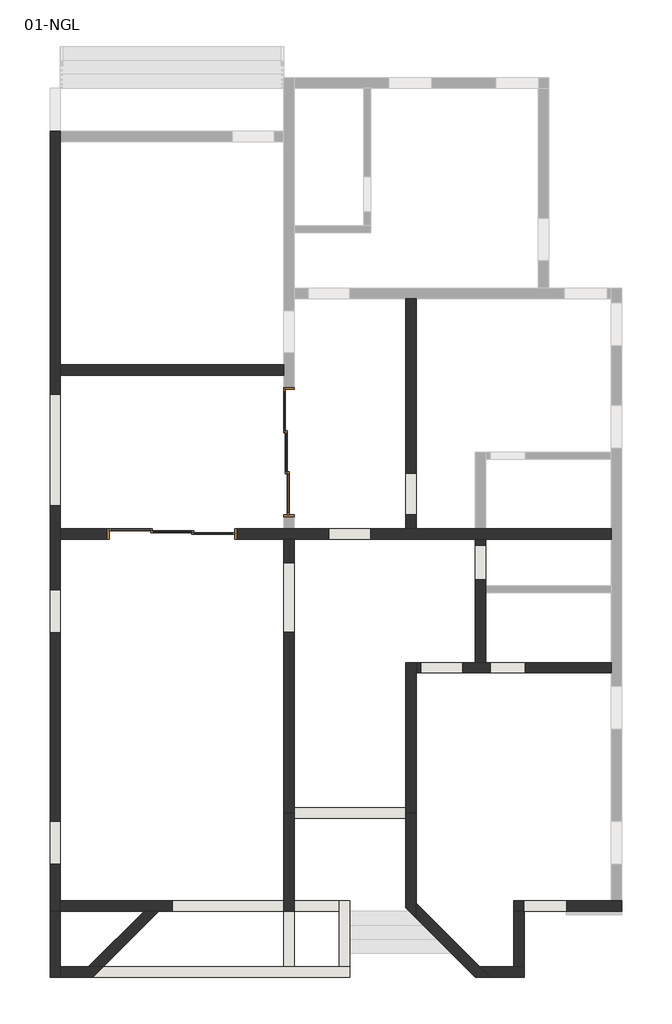
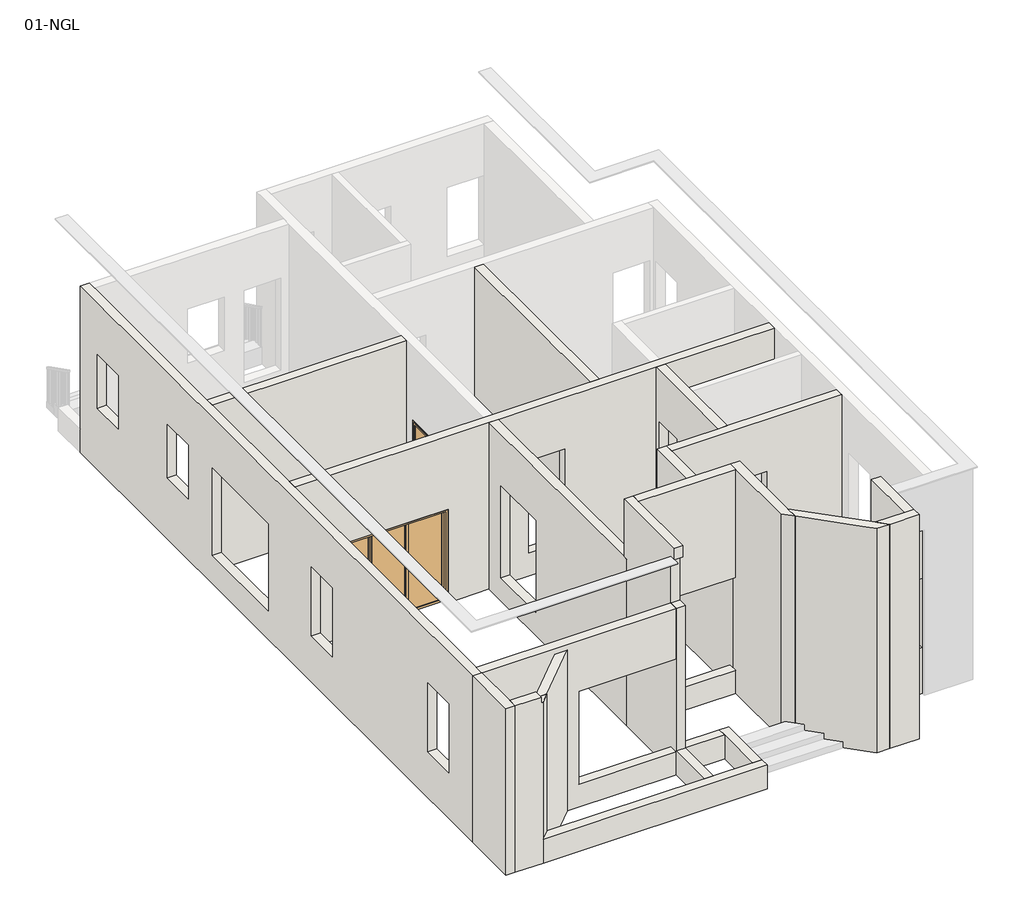
# One storey, part 1 of 2: 23 walls, 2 doors.
"""IFC4 building model written with IfcOpenShell, lengths in millimetres."""

from ifc_helpers import new_model, si_unit, frame, origin, origin_with_axes, place, context, project, spatial, polyline, outline, extrude, faceted_brep, transform, mapped, element, save
from components import d3_d2ac5bf4, d3_8cc66dcc

model = new_model("IFC4")

# Units and contexts
model_context = context("Model", 3, world=origin())
ifc_project = project(units=[si_unit("LENGTHUNIT", "METRE", prefix="MILLI")], contexts=[model_context])

# Site, building, storey
site = spatial("IfcSite", under=ifc_project)
building = spatial("IfcBuilding", under=site)
storey = spatial("IfcBuildingStorey", under=building, Name="01-NGL", Elevation=0.0)

# Doors
placement = place(None, origin())
d3_shape = d3_d2ac5bf4(model_context)
element("IfcDoor", 1, ObjectType="D3", at=placement, inside=storey, context=model_context, shape_type="MappedRepresentation", body=[
    mapped(d3_shape, transform((-3747.9564803, -2661.7684988, 0.0), x_axis=(0.0, -1.0, 0.0), y_axis=(1.0, 0.0, 0.0), z_axis=(0.0, 0.0, 1.0))),
])
d3_2_shape = d3_8cc66dcc(model_context)
element("IfcDoor", 2, ObjectType="D3", at=placement, inside=storey, context=model_context, shape_type="MappedRepresentation", body=[
    mapped(d3_2_shape, transform((-6346.2144815, -4510.0265, 0.0), x_axis=(1.0, 0.0, 0.0), y_axis=(0.0, 1.0, 0.0), z_axis=(0.0, 0.0, 1.0))),
])

# Walls
element("IfcWall", 3, ObjectType="01-225 wall", at=placement, inside=storey, context=model_context, shape_type="Brep", body=[
    faceted_brep([(-8660.4564803, -12622.5265, 0.0), (-8660.4564803, -12397.5265, 0.0), (-8660.4564803, -4622.5265, 0.0), (-8660.4564803, -4397.5265, 0.0), (-8660.4564803, -1097.5265, 0.0), (-8660.4564803, -872.5265, 0.0), (-8660.4564803, 3927.4735, 0.0), (-8660.4564803, 4152.4735, 0.0), (-8660.4564803, 4152.4735, 625.0), (-8660.4564803, 4152.4735, 4350.0), (-8660.4564803, 3927.4735, 4350.0), (-8660.4564803, -872.5265, 4350.0), (-8660.4564803, -1097.5265, 4350.0), (-8660.4564803, -4397.5265, 4350.0), (-8660.4564803, -4622.5265, 4350.0), (-8660.4564803, -12397.5265, 4350.0), (-8660.4564803, -12622.5265, 4350.0), (-8660.4564803, -11597.5265, 1200.0), (-8660.4564803, -11597.5265, 3000.0), (-8660.4564803, -10697.5265, 3000.0), (-8660.4564803, -10697.5265, 1200.0), (-8660.4564803, -6622.5265, 1200.0), (-8660.4564803, -6622.5265, 3000.0), (-8660.4564803, -5722.5265, 3000.0), (-8660.4564803, -5722.5265, 1200.0), (-8660.4564803, 3427.4735, 3000.0), (-8660.4564803, 3427.4735, 1600.0), (-8660.4564803, 2527.4735, 1600.0), (-8660.4564803, 2527.4735, 3000.0), (-8660.4564803, -472.5265, 1600.0), (-8660.4564803, -472.5265, 3000.0), (-8660.4564803, 427.4735, 3000.0), (-8660.4564803, 427.4735, 1600.0), (-8660.4564803, -1497.5265, 3025.0), (-8660.4564803, -1497.5265, 750.0), (-8660.4564803, -3897.5265, 750.0), (-8660.4564803, -3897.5265, 3025.0), (-8885.4564803, 4152.4735, 0.0), (-8885.4564803, -12622.5265, 0.0), (-8885.4564803, -12622.5265, 4350.0), (-8885.4564803, 4152.4735, 4350.0), (-8885.4564803, 4152.4735, 625.0), (-8885.4564803, -11597.5265, 3000.0), (-8885.4564803, -11597.5265, 1200.0), (-8885.4564803, -10697.5265, 1200.0), (-8885.4564803, -10697.5265, 3000.0), (-8885.4564803, -6622.5265, 3000.0), (-8885.4564803, -6622.5265, 1200.0), (-8885.4564803, -5722.5265, 1200.0), (-8885.4564803, -5722.5265, 3000.0), (-8885.4564803, 3427.4735, 1600.0), (-8885.4564803, 3427.4735, 3000.0), (-8885.4564803, 2527.4735, 3000.0), (-8885.4564803, 2527.4735, 1600.0), (-8885.4564803, -472.5265, 3000.0), (-8885.4564803, -472.5265, 1600.0), (-8885.4564803, 427.4735, 1600.0), (-8885.4564803, 427.4735, 3000.0), (-8885.4564803, -1497.5265, 750.0), (-8885.4564803, -1497.5265, 3025.0), (-8885.4564803, -3897.5265, 3025.0), (-8885.4564803, -3897.5265, 750.0)], [[[0, 1, 2, 3, 4, 5, 6, 7, 8, 9, 10, 11, 12, 13, 14, 15, 16], [17, 18, 19, 20], [21, 22, 23, 24], [25, 26, 27, 28], [29, 30, 31, 32], [33, 34, 35, 36]], [[37, 38, 39, 40, 41], [42, 43, 44, 45], [46, 47, 48, 49], [50, 51, 52, 53], [54, 55, 56, 57], [58, 59, 60, 61]], [[7, 6, 5, 4, 3, 2, 1, 0, 38, 37]], [[16, 15, 14, 13, 12, 11, 10, 9, 40, 39]], [[0, 16, 39, 38]], [[7, 37, 41, 40, 9, 8]], [[43, 42, 18, 17]], [[44, 43, 17, 20]], [[45, 44, 20, 19]], [[42, 45, 19, 18]], [[47, 46, 22, 21]], [[48, 47, 21, 24]], [[49, 48, 24, 23]], [[46, 49, 23, 22]], [[26, 25, 51, 50]], [[27, 26, 50, 53]], [[28, 27, 53, 52]], [[25, 28, 52, 51]], [[55, 54, 30, 29]], [[56, 55, 29, 32]], [[57, 56, 32, 31]], [[54, 57, 31, 30]], [[58, 34, 33, 59]], [[59, 33, 36, 60]], [[60, 36, 35, 61]], [[34, 58, 61, 35]]]),
])
element("IfcWall", 4, ObjectType="01-225 wall", at=placement, inside=storey, context=model_context, shape_type="Brep", body=[
    faceted_brep([(3189.5435197, -4622.5265, 4350.0), (489.5435197, -4622.5265, 4350.0), (264.5435197, -4622.5265, 4350.0), (-3635.4564803, -4622.5265, 4350.0), (-3860.4564803, -4622.5265, 4350.0), (-8660.4564803, -4622.5265, 4350.0), (-8660.4564803, -4622.5265, 0.0), (-7650.4564803, -4622.5265, 0.0), (-7650.4564803, -4622.5265, 2440.0), (-4870.4564803, -4622.5265, 2440.0), (-4870.4564803, -4622.5265, 0.0), (-3860.4564803, -4622.5265, 0.0), (-3635.4564803, -4622.5265, 0.0), (264.5435197, -4622.5265, 0.0), (489.5435197, -4622.5265, 0.0), (3189.5435197, -4622.5265, 0.0), (-2885.4564803, -4622.5265, 600.0), (-2885.4564803, -4622.5265, 3000.0), (-1985.4564803, -4622.5265, 3000.0), (-1985.4564803, -4622.5265, 600.0), (-8660.4564803, -4397.5265, 4350.0), (-3860.4564803, -4397.5265, 4350.0), (-3635.4564803, -4397.5265, 4350.0), (-1235.4564803, -4397.5265, 4350.0), (-1010.4564803, -4397.5265, 4350.0), (264.5435197, -4397.5265, 4350.0), (489.5435197, -4397.5265, 4350.0), (3189.5435197, -4397.5265, 4350.0), (3189.5435197, -4397.5265, 0.0), (489.5435197, -4397.5265, 0.0), (264.5435197, -4397.5265, 0.0), (-1010.4564803, -4397.5265, 0.0), (-1235.4564803, -4397.5265, 0.0), (-3635.4564803, -4397.5265, 0.0), (-3860.4564803, -4397.5265, 0.0), (-4870.4564803, -4397.5265, 0.0), (-4870.4564803, -4397.5265, 2440.0), (-7650.4564803, -4397.5265, 2440.0), (-7650.4564803, -4397.5265, 0.0), (-8660.4564803, -4397.5265, 0.0), (-2885.4564803, -4397.5265, 600.0), (-1985.4564803, -4397.5265, 600.0), (-1985.4564803, -4397.5265, 3000.0), (-2885.4564803, -4397.5265, 3000.0)], [[[0, 1, 2, 3, 4, 5, 6, 7, 8, 9, 10, 11, 12, 13, 14, 15], [16, 17, 18, 19]], [[20, 21, 22, 23, 24, 25, 26, 27, 28, 29, 30, 31, 32, 33, 34, 35, 36, 37, 38, 39], [40, 41, 42, 43]], [[6, 39, 38, 7]], [[28, 15, 14, 13, 12, 11, 10, 35, 34, 33, 32, 31, 30, 29]], [[5, 4, 3, 2, 1, 0, 27, 26, 25, 24, 23, 22, 21, 20]], [[6, 5, 20, 39]], [[0, 15, 28, 27]], [[17, 16, 40, 43]], [[18, 17, 43, 42]], [[19, 18, 42, 41]], [[16, 19, 41, 40]], [[37, 8, 7, 38]], [[8, 37, 36, 9]], [[9, 36, 35, 10]]]),
])
element("IfcWall", 5, ObjectType="01-225 wall", at=placement, inside=storey, context=model_context, shape_type="Brep", body=[
    faceted_brep([(-3860.4564803, -4622.5265, 0.0), (-3860.4564803, -10510.0265, 0.0), (-3860.4564803, -10510.0265, 4350.0), (-3860.4564803, -10397.5265, 4350.0), (-3860.4564803, -4622.5265, 4350.0), (-3860.4564803, -5122.5265, 600.0), (-3860.4564803, -5122.5265, 3000.0), (-3860.4564803, -6622.5265, 3000.0), (-3860.4564803, -6622.5265, 600.0), (-3635.4564803, -4622.5265, 0.0), (-3635.4564803, -4622.5265, 4350.0), (-3635.4564803, -10397.5265, 4350.0), (-3635.4564803, -10510.0265, 4350.0), (-3635.4564803, -10510.0265, 0.0), (-3635.4564803, -10397.5265, 0.0), (-3635.4564803, -5122.5265, 600.0), (-3635.4564803, -6622.5265, 600.0), (-3635.4564803, -6622.5265, 3000.0), (-3635.4564803, -5122.5265, 3000.0)], [[[0, 1, 2, 3, 4], [5, 6, 7, 8]], [[9, 10, 11, 12, 13, 14], [15, 16, 17, 18]], [[1, 0, 9, 14, 13]], [[2, 1, 13, 12]], [[4, 3, 2, 12, 11, 10]], [[0, 4, 10, 9]], [[6, 5, 15, 18]], [[7, 6, 18, 17]], [[8, 7, 17, 16]], [[5, 8, 16, 15]]]),
])
element("IfcWall", 6, ObjectType="01-225 wall", at=placement, inside=storey, context=model_context, shape_type="Brep", body=[
    faceted_brep([(-3860.4564803, -12397.5265, 0.0), (-8660.4564803, -12397.5265, 0.0), (-8660.4564803, -12397.5265, 4350.0), (-3860.4564803, -12397.5265, 4350.0), (-3860.4564803, -12397.5265, 3025.0), (-6260.4564803, -12397.5265, 3025.0), (-6260.4564803, -12397.5265, 600.0), (-3860.4564803, -12397.5265, 600.0), (-8660.4564803, -12622.5265, 0.0), (-6860.4564803, -12622.5265, 0.0), (-6542.2584287, -12622.5265, 0.0), (-3860.4564803, -12622.5265, 0.0), (-3860.4564803, -12622.5265, 600.0), (-6260.4564803, -12622.5265, 600.0), (-6260.4564803, -12622.5265, 3025.0), (-3860.4564803, -12622.5265, 3025.0), (-3860.4564803, -12622.5265, 4350.0), (-8660.4564803, -12622.5265, 4350.0)], [[[0, 1, 2, 3, 4, 5, 6, 7]], [[8, 9, 10, 11, 12, 13, 14, 15, 16, 17]], [[1, 0, 11, 10, 9, 8]], [[3, 2, 17, 16]], [[2, 1, 8, 17]], [[14, 5, 4, 15]], [[5, 14, 13, 6]], [[6, 13, 12, 7]], [[11, 0, 7, 12]], [[3, 16, 15, 4]]]),
])
element("IfcWall", 7, ObjectType="01-225 wall", at=placement, inside=storey, context=model_context, shape_type="Brep", body=[
    faceted_brep([(-3635.4564803, -10622.5265, 0.0), (-1235.4564803, -10622.5265, 0.0), (-1235.4564803, -10622.5265, 600.0), (-3635.4564803, -10622.5265, 600.0), (-1235.4564803, -10397.5265, 0.0), (-3635.4564803, -10397.5265, 0.0), (-3635.4564803, -10397.5265, 600.0), (-1235.4564803, -10397.5265, 600.0), (-3635.4564803, -10510.0265, 0.0), (-1235.4564803, -10510.0265, 0.0)], [[[0, 1, 2, 3]], [[4, 5, 6, 7]], [[1, 0, 8, 5, 4, 9]], [[3, 2, 7, 6]], [[1, 9, 4, 7, 2]], [[5, 8, 0, 3, 6]]]),
    faceted_brep([(-1235.4564803, -10622.5265, 5850.0), (-3635.4564803, -10622.5265, 5850.0), (-3635.4564803, -10622.5265, 3025.0), (-1235.4564803, -10622.5265, 3025.0), (-3635.4564803, -10397.5265, 5850.0), (-1235.4564803, -10397.5265, 5850.0), (-1235.4564803, -10397.5265, 4350.0), (-1235.4564803, -10397.5265, 3025.0), (-3635.4564803, -10397.5265, 3025.0), (-3635.4564803, -10397.5265, 4350.0)], [[[0, 1, 2, 3]], [[4, 5, 6, 7, 8, 9]], [[1, 0, 5, 4]], [[3, 2, 8, 7]], [[5, 0, 3, 7, 6]], [[1, 4, 9, 8, 2]]]),
])
element("IfcWall", 8, ObjectType="01-225 wall", at=placement, inside=storey, context=model_context, shape_type="SweptSolid", body=[
    extrude(outline(polyline([(552.4735, 0.0), (-4397.5265, 0.0), (-4397.5265, 4350.0), (552.4735, 4350.0), (552.4735, 0.0)]), holes=[polyline([(-4097.5265, 600.0), (-3197.5265, 600.0), (-3197.5265, 3000.0), (-4097.5265, 3000.0), (-4097.5265, 600.0)])]), frame((-1235.4564803, 0.0, 0.0), z_axis=(1.0, 0.0, 0.0), x_axis=(0.0, 1.0, 0.0)), (0.0, 0.0, 1.0), 225.0),
])
element("IfcWall", 9, ObjectType="01-225 wall", at=placement, inside=storey, context=model_context, shape_type="Brep", body=[
    faceted_brep([(1089.5435197, -12622.5265, 0.0), (1314.5435197, -12622.5265, 0.0), (3414.5435197, -12622.5265, 0.0), (3414.5435197, -12622.5265, 4350.0), (1314.5435197, -12622.5265, 4350.0), (1089.5435197, -12622.5265, 4350.0), (1314.5435197, -12622.5265, 3000.0), (2214.5435197, -12622.5265, 3000.0), (2214.5435197, -12622.5265, 1200.0), (1314.5435197, -12622.5265, 1200.0), (1089.5435197, -12397.5265, 0.0), (1089.5435197, -12397.5265, 4350.0), (1314.5435197, -12397.5265, 4350.0), (3189.5435197, -12397.5265, 4350.0), (3414.5435197, -12397.5265, 4350.0), (3414.5435197, -12397.5265, 0.0), (3189.5435197, -12397.5265, 0.0), (1314.5435197, -12397.5265, 3000.0), (1314.5435197, -12397.5265, 1200.0), (2214.5435197, -12397.5265, 1200.0), (2214.5435197, -12397.5265, 3000.0)], [[[0, 1, 2, 3, 4, 5], [6, 7, 8, 9]], [[10, 11, 12, 13, 14, 15, 16], [17, 18, 19, 20]], [[2, 1, 0, 10, 16, 15]], [[5, 4, 3, 14, 13, 12, 11]], [[3, 2, 15, 14]], [[0, 5, 11, 10]], [[18, 17, 6, 9]], [[19, 18, 9, 8]], [[20, 19, 8, 7]], [[17, 20, 7, 6]]]),
])
element("IfcWall", 10, ObjectType="01-225 wall", at=placement, inside=storey, context=model_context, shape_type="SweptSolid", body=[
    extrude(outline(polyline([(-3860.4564803, -1097.5265), (-8660.4564803, -1097.5265), (-8660.4564803, -872.5265), (-3860.4564803, -872.5265), (-3860.4564803, -1097.5265)])), origin_with_axes(), (0.0, 0.0, 1.0), 4350.0),
])
element("IfcWall", 11, ObjectType="01-225 wall", at=placement, inside=storey, context=model_context, shape_type="Brep", body=[
    faceted_brep([(-1010.4564803, -7497.5265, 0.0), (3189.5435197, -7497.5265, 0.0), (3189.5435197, -7497.5265, 4350.0), (-1010.4564803, -7497.5265, 4350.0), (-910.4564803, -7497.5265, 600.0), (-910.4564803, -7497.5265, 3000.0), (-10.4564803, -7497.5265, 3000.0), (-10.4564803, -7497.5265, 600.0), (589.5435197, -7497.5265, 600.0), (589.5435197, -7497.5265, 3000.0), (1339.5435197, -7497.5265, 3000.0), (1339.5435197, -7497.5265, 600.0), (-1010.4564803, -7272.5265, 0.0), (-1010.4564803, -7272.5265, 4350.0), (264.5435197, -7272.5265, 4350.0), (489.5435197, -7272.5265, 4350.0), (3189.5435197, -7272.5265, 4350.0), (3189.5435197, -7272.5265, 0.0), (489.5435197, -7272.5265, 0.0), (264.5435197, -7272.5265, 0.0), (-910.4564803, -7272.5265, 600.0), (-10.4564803, -7272.5265, 600.0), (-10.4564803, -7272.5265, 3000.0), (-910.4564803, -7272.5265, 3000.0), (589.5435197, -7272.5265, 600.0), (1339.5435197, -7272.5265, 600.0), (1339.5435197, -7272.5265, 3000.0), (589.5435197, -7272.5265, 3000.0)], [[[0, 1, 2, 3], [4, 5, 6, 7], [8, 9, 10, 11]], [[12, 13, 14, 15, 16, 17, 18, 19], [20, 21, 22, 23], [24, 25, 26, 27]], [[1, 0, 12, 19, 18, 17]], [[3, 2, 16, 15, 14, 13]], [[2, 1, 17, 16]], [[0, 3, 13, 12]], [[5, 4, 20, 23]], [[6, 5, 23, 22]], [[7, 6, 22, 21]], [[4, 7, 21, 20]], [[9, 8, 24, 27]], [[10, 9, 27, 26]], [[11, 10, 26, 25]], [[8, 11, 25, 24]]]),
])
element("IfcWall", 12, ObjectType="01-225 wall", at=placement, inside=storey, context=model_context, shape_type="Brep", body=[
    faceted_brep([(489.5435197, -7272.5265, 0.0), (489.5435197, -5772.5265, 0.0), (489.5435197, -5622.5265, 0.0), (489.5435197, -4622.5265, 0.0), (489.5435197, -4622.5265, 4350.0), (489.5435197, -5622.5265, 4350.0), (489.5435197, -5772.5265, 4350.0), (489.5435197, -7272.5265, 4350.0), (489.5435197, -4747.5265, 600.0), (489.5435197, -5497.5265, 600.0), (489.5435197, -5497.5265, 3000.0), (489.5435197, -4747.5265, 3000.0), (264.5435197, -7272.5265, 0.0), (264.5435197, -7272.5265, 4350.0), (264.5435197, -4622.5265, 4350.0), (264.5435197, -4622.5265, 0.0), (264.5435197, -4747.5265, 600.0), (264.5435197, -4747.5265, 3000.0), (264.5435197, -5497.5265, 3000.0), (264.5435197, -5497.5265, 600.0)], [[[0, 1, 2, 3, 4, 5, 6, 7], [8, 9, 10, 11]], [[12, 13, 14, 15], [16, 17, 18, 19]], [[3, 2, 1, 0, 12, 15]], [[7, 6, 5, 4, 14, 13]], [[4, 3, 15, 14]], [[0, 7, 13, 12]], [[17, 16, 8, 11]], [[18, 17, 11, 10]], [[19, 18, 10, 9]], [[16, 19, 9, 8]]]),
])
element("IfcWall", 13, ObjectType="01-225 wall", at=placement, inside=storey, context=model_context, shape_type="Brep", body=[
    faceted_brep([(-1235.4564803, -7272.5265, 0.0), (-1235.4564803, -10397.5265, 0.0), (-1235.4564803, -10510.0265, 0.0), (-1235.4564803, -10510.0265, 4350.0), (-1235.4564803, -10397.5265, 4350.0), (-1235.4564803, -7272.5265, 4350.0), (-1010.4564803, -7272.5265, 0.0), (-1010.4564803, -7272.5265, 4350.0), (-1010.4564803, -7497.5265, 4350.0), (-1010.4564803, -10397.5265, 4350.0), (-1010.4564803, -10510.0265, 4350.0), (-1010.4564803, -10510.0265, 0.0), (-1010.4564803, -7497.5265, 0.0)], [[[0, 1, 2, 3, 4, 5]], [[6, 7, 8, 9, 10, 11, 12]], [[2, 1, 0, 6, 12, 11]], [[3, 2, 11, 10]], [[5, 4, 3, 10, 9, 8, 7]], [[0, 5, 7, 6]]]),
])
element("IfcWall", 14, ObjectType="01-225 wall", at=placement, inside=storey, context=model_context, shape_type="Brep", body=[
    faceted_brep([(-8885.4564803, -12622.5265, 0.0), (-8885.4564803, -14047.5265, 0.0), (-8885.4564803, -14047.5265, 4350.0), (-8885.4564803, -12622.5265, 4350.0), (-8660.4564803, -12622.5265, 0.0), (-8660.4564803, -12622.5265, 4350.0), (-8660.4564803, -13822.5265, 4350.0), (-8660.4564803, -14047.5265, 4350.0), (-8660.4564803, -14047.5265, 0.0), (-8660.4564803, -13822.5265, 0.0)], [[[0, 1, 2, 3]], [[4, 5, 6, 7, 8, 9]], [[1, 0, 4, 9, 8]], [[3, 2, 7, 6, 5]], [[0, 3, 5, 4]], [[2, 1, 8, 7]]]),
])
element("IfcWall", 15, ObjectType="01-225 wall", at=placement, inside=storey, context=model_context, shape_type="Brep", body=[
    faceted_brep([(-8660.4564803, -14047.5265, 0.0), (-7967.2584287, -14047.5265, 0.0), (-7967.2584287, -14047.5265, 625.0), (-7967.2584287, -14047.5265, 3900.0), (-7967.2584287, -14047.5265, 4200.0), (-8013.8574545, -14047.5265, 4200.0), (-8013.8574545, -14047.5265, 4350.0), (-8660.4564803, -14047.5265, 4350.0), (-8660.4564803, -13822.5265, 0.0), (-8660.4564803, -13822.5265, 4350.0), (-8013.8574545, -13822.5265, 4350.0), (-8013.8574545, -13822.5265, 4200.0), (-7742.2584287, -13822.5265, 4200.0), (-7742.2584287, -13822.5265, 3900.0), (-7742.2584287, -13822.5265, 625.0), (-7742.2584287, -13822.5265, 0.0), (-8060.4564803, -13822.5265, 0.0)], [[[0, 1, 2, 3, 4, 5, 6, 7]], [[8, 9, 10, 11, 12, 13, 14, 15, 16]], [[1, 0, 8, 16, 15]], [[7, 6, 10, 9]], [[0, 7, 9, 8]], [[6, 5, 11, 10]], [[11, 5, 4, 12]], [[1, 15, 14, 13, 12, 4, 3, 2]]]),
])
element("IfcWall", 16, ObjectType="01-225 wall", at=placement, inside=storey, context=model_context, shape_type="Brep", body=[
    faceted_brep([(-7742.2584287, -13822.5265, 4200.0), (-7742.2584287, -13822.5265, 0.0), (-6542.2584287, -12622.5265, 0.0), (-6542.2584287, -12622.5265, 4200.0), (-8060.4564803, -13822.5265, 0.0), (-8060.4564803, -13822.5265, 4200.0), (-6860.4564803, -12622.5265, 4200.0), (-6860.4564803, -12622.5265, 0.0), (-8013.8574545, -13822.5265, 4200.0)], [[[0, 1, 2, 3]], [[4, 5, 6, 7]], [[2, 1, 4, 7]], [[0, 3, 6, 5, 8]], [[3, 2, 7, 6]], [[0, 8, 5, 4, 1]]]),
])
element("IfcWall", 17, ObjectType="01-225 wall", at=placement, inside=storey, context=model_context, shape_type="Brep", body=[
    faceted_brep([(-7967.2584287, -14047.5265, 0.0), (-2435.4564803, -14047.5265, 0.0), (-2435.4564803, -14047.5265, 625.0), (-7967.2584287, -14047.5265, 625.0), (-7742.2584287, -13822.5265, 0.0), (-7742.2584287, -13822.5265, 625.0), (-3860.4564803, -13822.5265, 625.0), (-3635.4564803, -13822.5265, 625.0), (-2660.4564803, -13822.5265, 625.0), (-2435.4564803, -13822.5265, 625.0), (-2435.4564803, -13822.5265, 0.0), (-2660.4564803, -13822.5265, 0.0), (-3635.4564803, -13822.5265, 0.0), (-3860.4564803, -13822.5265, 0.0)], [[[0, 1, 2, 3]], [[4, 5, 6, 7, 8, 9, 10, 11, 12, 13]], [[1, 0, 4, 13, 12, 11, 10]], [[3, 2, 9, 8, 7, 6, 5]], [[0, 3, 5, 4]], [[2, 1, 10, 9]]]),
])
element("IfcWall", 18, ObjectType="01-225 wall", at=placement, inside=storey, context=model_context, shape_type="Brep", body=[
    faceted_brep([(-2435.4564803, -13822.5265, 0.0), (-2435.4564803, -12397.5265, 0.0), (-2435.4564803, -12397.5265, 625.0), (-2435.4564803, -13822.5265, 625.0), (-2660.4564803, -13822.5265, 0.0), (-2660.4564803, -13822.5265, 625.0), (-2660.4564803, -12622.5265, 625.0), (-2660.4564803, -12397.5265, 625.0), (-2660.4564803, -12397.5265, 0.0), (-2660.4564803, -12622.5265, 0.0)], [[[0, 1, 2, 3]], [[4, 5, 6, 7, 8, 9]], [[1, 0, 4, 9, 8]], [[3, 2, 7, 6, 5]], [[0, 3, 5, 4]], [[2, 1, 8, 7]]]),
])
element("IfcWall", 19, ObjectType="01-225 wall", at=placement, inside=storey, context=model_context, shape_type="Brep", body=[
    faceted_brep([(582.7415713, -14047.5265, 5850.0), (582.7415713, -14047.5265, 0.0), (1314.5435197, -14047.5265, 0.0), (1314.5435197, -14047.5265, 5850.0), (357.7415713, -13822.5265, 0.0), (357.7415713, -13822.5265, 5850.0), (1089.5435197, -13822.5265, 5850.0), (1314.5435197, -13822.5265, 5850.0), (1314.5435197, -13822.5265, 0.0), (1089.5435197, -13822.5265, 0.0)], [[[0, 1, 2, 3]], [[4, 5, 6, 7, 8, 9]], [[2, 1, 4, 9, 8]], [[0, 3, 7, 6, 5]], [[3, 2, 8, 7]], [[0, 5, 4, 1]]]),
])
element("IfcWall", 20, ObjectType="01-225 wall", at=placement, inside=storey, context=model_context, shape_type="Brep", body=[
    faceted_brep([(1314.5435197, -13822.5265, 0.0), (1314.5435197, -12622.5265, 0.0), (1314.5435197, -12622.5265, 1200.0), (1314.5435197, -12622.5265, 3000.0), (1314.5435197, -12622.5265, 4350.0), (1314.5435197, -12397.5265, 4350.0), (1314.5435197, -12397.5265, 5550.0), (1314.5435197, -12397.5265, 5850.0), (1314.5435197, -13822.5265, 5850.0), (1089.5435197, -13822.5265, 0.0), (1089.5435197, -13822.5265, 5850.0), (1089.5435197, -12397.5265, 5850.0), (1089.5435197, -12397.5265, 4350.0), (1089.5435197, -12622.5265, 4350.0), (1089.5435197, -12622.5265, 0.0)], [[[0, 1, 2, 3, 4, 5, 6, 7, 8]], [[9, 10, 11, 12, 13, 14]], [[1, 0, 9, 14]], [[8, 7, 11, 10]], [[0, 8, 10, 9]], [[12, 5, 4, 13]], [[4, 3, 2, 1, 14, 13]], [[7, 6, 5, 12, 11]]]),
])
element("IfcWall", 21, ObjectType="01-225 wall", at=placement, inside=storey, context=model_context, shape_type="Brep", body=[
    faceted_brep([(582.7415713, -14047.5265, 5850.0), (582.7415713, -14047.5265, 0.0), (357.7415713, -13822.5265, 0.0), (-1010.4564803, -12454.3284484, 0.0), (-1010.4564803, -12454.3284484, 5850.0), (357.7415713, -13822.5265, 5850.0), (264.5435197, -14047.5265, 0.0), (264.5435197, -14047.5265, 5250.0), (264.5435197, -14047.5265, 5850.0), (39.5435197, -13822.5265, 5850.0), (-1010.4564803, -12772.5265, 5850.0), (-1010.4564803, -12772.5265, 0.0)], [[[0, 1, 2, 3, 4, 5]], [[6, 7, 8, 9, 10, 11]], [[3, 2, 1, 6, 11]], [[0, 5, 4, 10, 9, 8]], [[4, 3, 11, 10]], [[0, 8, 7, 6, 1]]]),
])
element("IfcWall", 22, ObjectType="01-225 wall", at=placement, inside=storey, context=model_context, shape_type="SweptSolid", body=[
    extrude(outline(polyline([(-2660.4564803, -12622.5265), (-3635.4564803, -12622.5265), (-3635.4564803, -12397.5265), (-2660.4564803, -12397.5265), (-2660.4564803, -12622.5265)])), origin_with_axes(), (0.0, 0.0, 1.0), 625.0),
])
element("IfcWall", 23, ObjectType="01-225 wall", at=placement, inside=storey, context=model_context, shape_type="SweptSolid", body=[
    extrude(outline(polyline([(-3635.4564803, -12622.5265), (-3635.4564803, -13822.5265), (-3860.4564803, -13822.5265), (-3860.4564803, -12622.5265), (-3635.4564803, -12622.5265)])), origin_with_axes(), (0.0, 0.0, 1.0), 625.0),
])
element("IfcWall", 24, ObjectType="01-225 wall", at=placement, inside=storey, context=model_context, shape_type="Brep", body=[
    faceted_brep([(-3860.4564803, -10510.0265, 0.0), (-3860.4564803, -12397.5265, 0.0), (-3860.4564803, -12622.5265, 0.0), (-3860.4564803, -12622.5265, 600.0), (-3860.4564803, -12622.5265, 625.0), (-3860.4564803, -12622.5265, 3025.0), (-3860.4564803, -12622.5265, 4350.0), (-3860.4564803, -12397.5265, 4350.0), (-3860.4564803, -12397.5265, 5250.0), (-3860.4564803, -12397.5265, 5550.0), (-3860.4564803, -12510.0265, 5550.0), (-3860.4564803, -12510.0265, 5850.0), (-3860.4564803, -10397.5265, 5850.0), (-3860.4564803, -10397.5265, 4350.0), (-3860.4564803, -10510.0265, 4350.0), (-3635.4564803, -10510.0265, 0.0), (-3635.4564803, -10510.0265, 4350.0), (-3635.4564803, -10397.5265, 4350.0), (-3635.4564803, -10397.5265, 5850.0), (-3635.4564803, -10622.5265, 5850.0), (-3635.4564803, -12510.0265, 5850.0), (-3635.4564803, -12510.0265, 5550.0), (-3635.4564803, -12397.5265, 5550.0), (-3635.4564803, -12397.5265, 5250.0), (-3635.4564803, -12397.5265, 4350.0), (-3635.4564803, -12622.5265, 4350.0), (-3635.4564803, -12622.5265, 625.0), (-3635.4564803, -12622.5265, 0.0), (-3635.4564803, -12397.5265, 0.0), (-3635.4564803, -10622.5265, 0.0)], [[[0, 1, 2, 3, 4, 5, 6, 7, 8, 9, 10, 11, 12, 13, 14]], [[15, 16, 17, 18, 19, 20, 21, 22, 23, 24, 25, 26, 27, 28, 29]], [[2, 1, 0, 15, 29, 28, 27]], [[12, 11, 20, 19, 18]], [[0, 14, 16, 15]], [[13, 17, 16, 14]], [[13, 12, 18, 17]], [[24, 7, 6, 25]], [[2, 27, 26, 25, 6, 5, 4, 3]], [[11, 10, 21, 20]], [[21, 10, 9, 22]], [[9, 8, 7, 24, 23, 22]]]),
])
element("IfcWall", 25, ObjectType="01-225 wall", at=placement, inside=storey, context=model_context, shape_type="Brep", body=[
    faceted_brep([(-1235.4564803, -10510.0265, 0.0), (-1235.4564803, -10622.5265, 0.0), (-1235.4564803, -12547.5265, 0.0), (-1235.4564803, -12547.5265, 5850.0), (-1235.4564803, -10622.5265, 5850.0), (-1235.4564803, -10397.5265, 5850.0), (-1235.4564803, -10397.5265, 4350.0), (-1235.4564803, -10510.0265, 4350.0), (-1010.4564803, -10510.0265, 0.0), (-1010.4564803, -10510.0265, 4350.0), (-1010.4564803, -10397.5265, 4350.0), (-1010.4564803, -10397.5265, 5850.0), (-1010.4564803, -12454.3284484, 5850.0), (-1010.4564803, -12772.5265, 5850.0), (-1010.4564803, -12772.5265, 0.0), (-1010.4564803, -12454.3284484, 0.0)], [[[0, 1, 2, 3, 4, 5, 6, 7]], [[8, 9, 10, 11, 12, 13, 14, 15]], [[2, 1, 0, 8, 15, 14]], [[5, 4, 3, 13, 12, 11]], [[3, 2, 14, 13]], [[0, 7, 9, 8]], [[6, 10, 9, 7]], [[6, 5, 11, 10]]]),
])

save(model, "model.ifc")

# Revit data of these elements
# Type "D3"
#   Type Mark = "52"
#   Operation = "UserDefined"
#   Width = 2700 mm
#   Thickness = 40 mm
#   Rough Width = 2780 mm
#   Rough Height = 2440 mm
#   Panel Width = 927.5 mm
#   Panel Frame = 55 mm
#   Height = 2400 mm
#   Frame Depth = 40 mm
#   Glass Material = Sliding Door Glass
#   Frame Material = Sliding Door Frame
#   Function = (empty or 0)
# Type "01-225 wall"
#   Description = "Generic Wall (Material By Category), 200mm thick"
#   Assembly Code = "B2010"
#   Type Mark = "G06"
#   Layers, outside or top first: 225 mm "01-225 wall paint" (function 1)
# Elements 1, 2 (IfcDoor, "D3")
#   Phase Created = New Construction
#   Materials on its faces: "Sliding Door Frame", "Sliding Door Glass"
# Elements 3, 4, 5, 6, 8, 9, 10, 11, 12, 13, 14, 15 (IfcWall, "01-225 wall")
#   Top Offset = 0 mm
#   Base Offset = 0 mm
#   wall height = 4350 mm
#   Phase Created = New Construction
#   Base Constraint = 01-NGL
#   Top Constraint = 05-ROOF
#   Materials on its faces: "01-225 wall paint"
# Elements 7, 19, 20, 21, 24, 25 (IfcWall, "01-225 wall")
#   Top Offset = 300 mm
#   Base Offset = 0 mm
#   wall height = 5850 mm
#   Phase Created = New Construction
#   Base Constraint = 01-NGL
#   Top Constraint = 06-PARAPET
#   Materials on its faces: "01-225 wall paint"
# Element 16 (IfcWall, "01-225 wall")
#   Top Offset = -150 mm
#   Base Offset = 0 mm
#   wall height = 4200 mm
#   Phase Created = New Construction
#   Base Constraint = 01-NGL
#   Top Constraint = 05-ROOF
#   Materials on its faces: "01-225 wall paint"
# Elements 17, 18, 22, 23 (IfcWall, "01-225 wall")
#   Top Offset = 25 mm
#   Base Offset = 0 mm
#   wall height = 625 mm
#   Phase Created = New Construction
#   Base Constraint = 01-NGL
#   Top Constraint = 02-DPC
#   Materials on its faces: "01-225 wall paint"
# Materials
#   "Sliding Door Glass": colour RGB 247 247 247, transparency 0.68
#   "Sliding Door Frame": colour RGB 160 107 8, transparency 0
#   "01-225 wall paint": class "Generic", colour RGB 242 242 255, transparency 0, Cost = 0
